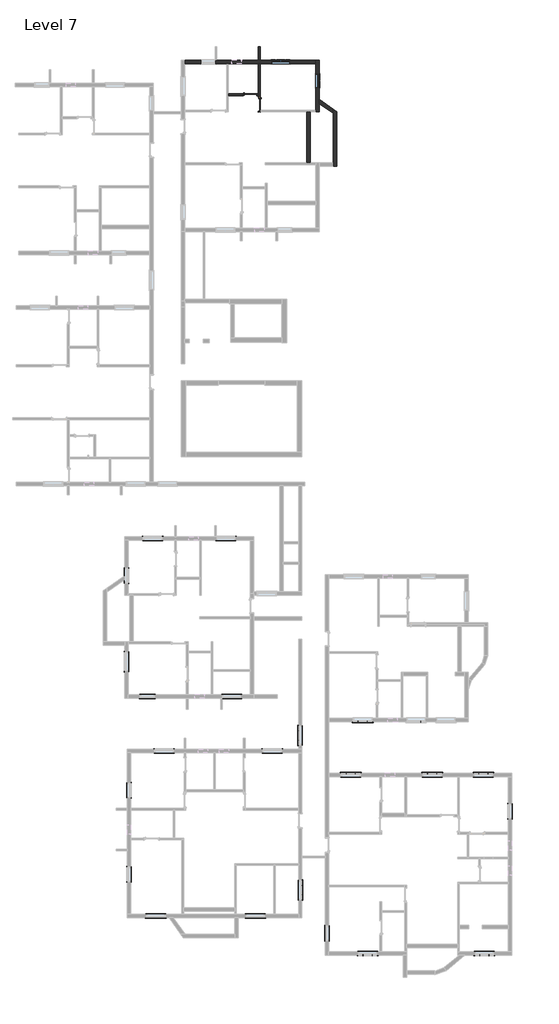
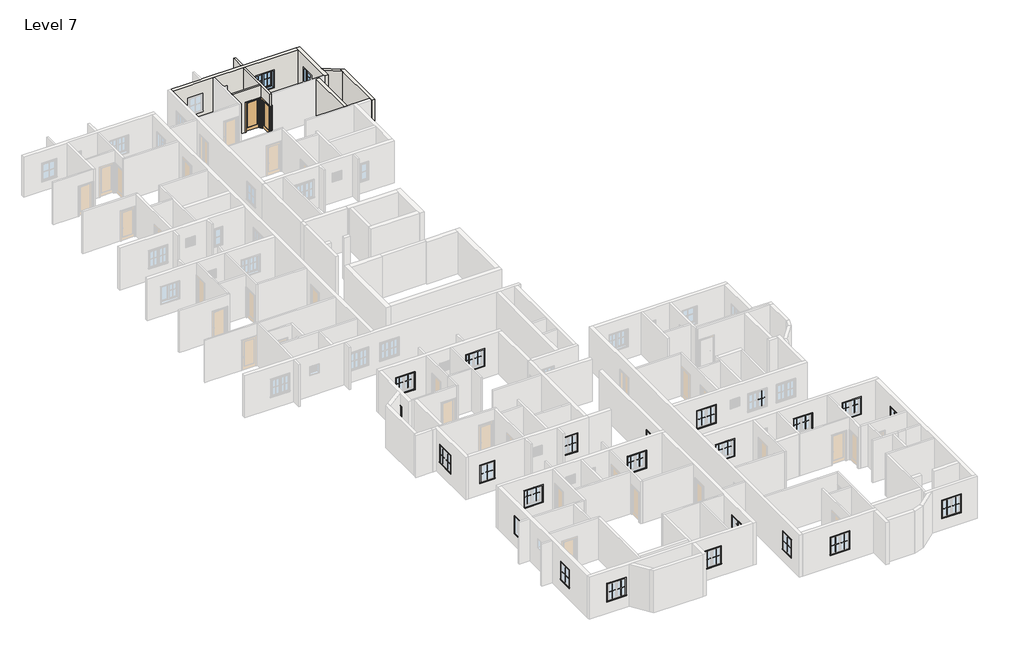
# One storey, part 6 of 7: 82 proxies, 8 walls, 2 doors, 2 windows.
"""IFC4 building model written with IfcOpenShell, lengths in millimetres."""

from ifc_helpers import new_model, si_unit, frame, origin, place, context, project, spatial, polyline, outline, extrude, faceted_brep, transform, mapped, element, save
from components import muntin_pattern_2x2_muntin_pattern_2x2_95b57395, muntin_pattern_2x2_muntin_pattern_2x2_4dfeb3f3, muntin_pattern_2x2_muntin_pattern_2x2_e852a7e4, trim_window_exterior_flat_with_sill_e4b28ec3, trim_window_exterior_flat_with_sill_7cfdd449, trim_window_interior_flat_picture_frame_39ff4276, trim_window_interior_flat_picture_frame_f1e0b15b, door_3c6ab76a, window_272f20d6, window_casement_double_4_x_4_af3140d2

model = new_model("IFC4")

# Units and contexts
model_context = context("Model", 3, world=origin())
ifc_project = project(units=[si_unit("LENGTHUNIT", "METRE", prefix="MILLI")], contexts=[model_context])

# Site, building, storey
site = spatial("IfcSite", under=ifc_project)
building = spatial("IfcBuilding", under=site)
storey = spatial("IfcBuildingStorey", under=building, Name="Level 7", Elevation=9601.2)

# Proxies
placement = place(None, origin())
muntin_pattern_2x2_muntin_pattern_2x2_shape = muntin_pattern_2x2_muntin_pattern_2x2_95b57395(model_context)
element("IfcBuildingElementProxy", 1, Name="Muntin Pattern_2x2 : Muntin Pattern_2x2", ObjectType="Muntin Pattern_2x2 : Muntin Pattern_2x2", at=placement, inside=storey, context=model_context, shape_type="MappedRepresentation", body=[
    mapped(muntin_pattern_2x2_muntin_pattern_2x2_shape, transform((17627.3240531, -20041.5997229, 10585.45), x_axis=(0.0, 1.0, 0.0), y_axis=(-1.0, 0.0, 0.0), z_axis=(0.0, 0.0, 1.0))),
])
element("IfcBuildingElementProxy", 2, Name="Muntin Pattern_2x2 : Muntin Pattern_2x2", ObjectType="Muntin Pattern_2x2 : Muntin Pattern_2x2", at=placement, inside=storey, context=model_context, shape_type="MappedRepresentation", body=[
    mapped(muntin_pattern_2x2_muntin_pattern_2x2_shape, transform((5625.8240531, -28048.9497229, 10585.45), x_axis=(0.0, 1.0, 0.0), y_axis=(-1.0, 0.0, 0.0), z_axis=(0.0, 0.0, 1.0))),
])
element("IfcBuildingElementProxy", 3, Name="Muntin Pattern_2x2 : Muntin Pattern_2x2", ObjectType="Muntin Pattern_2x2 : Muntin Pattern_2x2", at=placement, inside=storey, context=model_context, shape_type="MappedRepresentation", body=[
    mapped(muntin_pattern_2x2_muntin_pattern_2x2_shape, transform((-7378.9759469, -24172.9363256, 10585.45), x_axis=(0.0, 1.0, 0.0), y_axis=(-1.0, 0.0, 0.0), z_axis=(0.0, 0.0, 1.0))),
])
element("IfcBuildingElementProxy", 4, Name="Muntin Pattern_2x2 : Muntin Pattern_2x2", ObjectType="Muntin Pattern_2x2 : Muntin Pattern_2x2", at=placement, inside=storey, context=model_context, shape_type="MappedRepresentation", body=[
    mapped(muntin_pattern_2x2_muntin_pattern_2x2_shape, transform((-7169.4259469, -18656.0038828, 10585.45), x_axis=(0.0, -1.0, 0.0), y_axis=(1.0, 0.0, 0.0), z_axis=(0.0, 0.0, 1.0))),
])
element("IfcBuildingElementProxy", 5, Name="Muntin Pattern_2x2 : Muntin Pattern_2x2", ObjectType="Muntin Pattern_2x2 : Muntin Pattern_2x2", at=placement, inside=storey, context=model_context, shape_type="MappedRepresentation", body=[
    mapped(muntin_pattern_2x2_muntin_pattern_2x2_shape, transform((-6067.7009469, -12594.9288828, 10585.45), x_axis=(-1.0, 0.0, 0.0), y_axis=(0.0, -1.0, 0.0), z_axis=(0.0, 0.0, 1.0))),
])
element("IfcBuildingElementProxy", 6, Name="Muntin Pattern_2x2 : Muntin Pattern_2x2", ObjectType="Muntin Pattern_2x2 : Muntin Pattern_2x2", at=placement, inside=storey, context=model_context, shape_type="MappedRepresentation", body=[
    mapped(muntin_pattern_2x2_muntin_pattern_2x2_shape, transform((-7334.5259469, -4559.0038828, 10585.45), x_axis=(0.0, -1.0, 0.0), y_axis=(1.0, 0.0, 0.0), z_axis=(0.0, 0.0, 1.0))),
])
muntin_pattern_2x2_muntin_pattern_2x2_2_shape = muntin_pattern_2x2_muntin_pattern_2x2_4dfeb3f3(model_context)
element("IfcBuildingElementProxy", 7, Name="Muntin Pattern_2x2 : Muntin Pattern_2x2", ObjectType="Muntin Pattern_2x2 : Muntin Pattern_2x2", at=placement, inside=storey, context=model_context, shape_type="MappedRepresentation", body=[
    mapped(muntin_pattern_2x2_muntin_pattern_2x2_2_shape, transform((11869.4615531, -14158.3247229, 10585.45), x_axis=(-1.0, 0.0, 0.0), y_axis=(0.0, -1.0, 0.0), z_axis=(0.0, 0.0, 1.0))),
])
element("IfcBuildingElementProxy", 8, Name="Muntin Pattern_2x2 : Muntin Pattern_2x2", ObjectType="Muntin Pattern_2x2 : Muntin Pattern_2x2", at=placement, inside=storey, context=model_context, shape_type="MappedRepresentation", body=[
    mapped(muntin_pattern_2x2_muntin_pattern_2x2_2_shape, transform((8364.2615531, -14158.3247229, 10585.45), x_axis=(-1.0, 0.0, 0.0), y_axis=(0.0, -1.0, 0.0), z_axis=(0.0, 0.0, 1.0))),
])
element("IfcBuildingElementProxy", 9, Name="Muntin Pattern_2x2 : Muntin Pattern_2x2", ObjectType="Muntin Pattern_2x2 : Muntin Pattern_2x2", at=placement, inside=storey, context=model_context, shape_type="MappedRepresentation", body=[
    mapped(muntin_pattern_2x2_muntin_pattern_2x2_2_shape, transform((6976.7865531, -17530.1747229, 10585.45), x_axis=(1.0, 0.0, 0.0), y_axis=(0.0, 1.0, 0.0), z_axis=(0.0, 0.0, 1.0))),
])
element("IfcBuildingElementProxy", 10, Name="Muntin Pattern_2x2 : Muntin Pattern_2x2", ObjectType="Muntin Pattern_2x2 : Muntin Pattern_2x2", at=placement, inside=storey, context=model_context, shape_type="MappedRepresentation", body=[
    mapped(muntin_pattern_2x2_muntin_pattern_2x2_2_shape, transform((12323.4865531, -17530.1747229, 10585.45), x_axis=(1.0, 0.0, 0.0), y_axis=(0.0, 1.0, 0.0), z_axis=(0.0, 0.0, 1.0))),
])
element("IfcBuildingElementProxy", 11, Name="Muntin Pattern_2x2 : Muntin Pattern_2x2", ObjectType="Muntin Pattern_2x2 : Muntin Pattern_2x2", at=placement, inside=storey, context=model_context, shape_type="MappedRepresentation", body=[
    mapped(muntin_pattern_2x2_muntin_pattern_2x2_2_shape, transform((15682.6365531, -17530.1747229, 10585.45), x_axis=(1.0, 0.0, 0.0), y_axis=(0.0, 1.0, 0.0), z_axis=(0.0, 0.0, 1.0))),
])
element("IfcBuildingElementProxy", 12, Name="Muntin Pattern_2x2 : Muntin Pattern_2x2", ObjectType="Muntin Pattern_2x2 : Muntin Pattern_2x2", at=placement, inside=storey, context=model_context, shape_type="MappedRepresentation", body=[
    mapped(muntin_pattern_2x2_muntin_pattern_2x2_2_shape, transform((16349.3865531, -29474.5247229, 10585.45), x_axis=(-1.0, 0.0, 0.0), y_axis=(0.0, -1.0, 0.0), z_axis=(0.0, 0.0, 1.0))),
])
element("IfcBuildingElementProxy", 13, Name="Muntin Pattern_2x2 : Muntin Pattern_2x2", ObjectType="Muntin Pattern_2x2 : Muntin Pattern_2x2", at=placement, inside=storey, context=model_context, shape_type="MappedRepresentation", body=[
    mapped(muntin_pattern_2x2_muntin_pattern_2x2_2_shape, transform((8694.4615531, -29474.5247229, 10585.45), x_axis=(-1.0, 0.0, 0.0), y_axis=(0.0, -1.0, 0.0), z_axis=(0.0, 0.0, 1.0))),
])
element("IfcBuildingElementProxy", 14, Name="Muntin Pattern_2x2 : Muntin Pattern_2x2", ObjectType="Muntin Pattern_2x2 : Muntin Pattern_2x2", at=placement, inside=storey, context=model_context, shape_type="MappedRepresentation", body=[
    mapped(muntin_pattern_2x2_muntin_pattern_2x2_2_shape, transform((4070.0740531, -24902.8163828, 10585.45), x_axis=(0.0, -1.0, 0.0), y_axis=(1.0, 0.0, 0.0), z_axis=(0.0, 0.0, 1.0))),
])
element("IfcBuildingElementProxy", 15, Name="Muntin Pattern_2x2 : Muntin Pattern_2x2", ObjectType="Muntin Pattern_2x2 : Muntin Pattern_2x2", at=placement, inside=storey, context=model_context, shape_type="MappedRepresentation", body=[
    mapped(muntin_pattern_2x2_muntin_pattern_2x2_2_shape, transform((1325.2865531, -26996.7288828, 10585.45), x_axis=(-1.0, 0.0, 0.0), y_axis=(0.0, -1.0, 0.0), z_axis=(0.0, 0.0, 1.0))),
])
element("IfcBuildingElementProxy", 16, Name="Muntin Pattern_2x2 : Muntin Pattern_2x2", ObjectType="Muntin Pattern_2x2 : Muntin Pattern_2x2", at=placement, inside=storey, context=model_context, shape_type="MappedRepresentation", body=[
    mapped(muntin_pattern_2x2_muntin_pattern_2x2_2_shape, transform((-5208.8634469, -26996.7288828, 10585.45), x_axis=(-1.0, 0.0, 0.0), y_axis=(0.0, -1.0, 0.0), z_axis=(0.0, 0.0, 1.0))),
])
element("IfcBuildingElementProxy", 17, Name="Muntin Pattern_2x2 : Muntin Pattern_2x2", ObjectType="Muntin Pattern_2x2 : Muntin Pattern_2x2", at=placement, inside=storey, context=model_context, shape_type="MappedRepresentation", body=[
    mapped(muntin_pattern_2x2_muntin_pattern_2x2_2_shape, transform((1823.7615531, -15966.7788828, 10585.45), x_axis=(1.0, 0.0, 0.0), y_axis=(0.0, 1.0, 0.0), z_axis=(0.0, 0.0, 1.0))),
])
element("IfcBuildingElementProxy", 18, Name="Muntin Pattern_2x2 : Muntin Pattern_2x2", ObjectType="Muntin Pattern_2x2 : Muntin Pattern_2x2", at=placement, inside=storey, context=model_context, shape_type="MappedRepresentation", body=[
    mapped(muntin_pattern_2x2_muntin_pattern_2x2_2_shape, transform((-5272.3634469, -15966.7788828, 10585.45), x_axis=(1.0, 0.0, 0.0), y_axis=(0.0, 1.0, 0.0), z_axis=(0.0, 0.0, 1.0))),
])
element("IfcBuildingElementProxy", 19, Name="Muntin Pattern_2x2 : Muntin Pattern_2x2", ObjectType="Muntin Pattern_2x2 : Muntin Pattern_2x2", at=placement, inside=storey, context=model_context, shape_type="MappedRepresentation", body=[
    mapped(muntin_pattern_2x2_muntin_pattern_2x2_2_shape, transform((3860.5240531, -15358.7663828, 10585.45), x_axis=(0.0, 1.0, 0.0), y_axis=(-1.0, 0.0, 0.0), z_axis=(0.0, 0.0, 1.0))),
])
element("IfcBuildingElementProxy", 20, Name="Muntin Pattern_2x2 : Muntin Pattern_2x2", ObjectType="Muntin Pattern_2x2 : Muntin Pattern_2x2", at=placement, inside=storey, context=model_context, shape_type="MappedRepresentation", body=[
    mapped(muntin_pattern_2x2_muntin_pattern_2x2_2_shape, transform((-239.9884469, -12594.9288828, 10585.45), x_axis=(-1.0, 0.0, 0.0), y_axis=(0.0, -1.0, 0.0), z_axis=(0.0, 0.0, 1.0))),
])
element("IfcBuildingElementProxy", 21, Name="Muntin Pattern_2x2 : Muntin Pattern_2x2", ObjectType="Muntin Pattern_2x2 : Muntin Pattern_2x2", at=placement, inside=storey, context=model_context, shape_type="MappedRepresentation", body=[
    mapped(muntin_pattern_2x2_muntin_pattern_2x2_2_shape, transform((-7544.0759469, -10513.7163828, 10585.45), x_axis=(0.0, 1.0, 0.0), y_axis=(-1.0, 0.0, 0.0), z_axis=(0.0, 0.0, 1.0))),
])
element("IfcBuildingElementProxy", 22, Name="Muntin Pattern_2x2 : Muntin Pattern_2x2", ObjectType="Muntin Pattern_2x2 : Muntin Pattern_2x2", at=placement, inside=storey, context=model_context, shape_type="MappedRepresentation", body=[
    mapped(muntin_pattern_2x2_muntin_pattern_2x2_2_shape, transform((-6021.6634469, -2022.1788828, 10585.45), x_axis=(1.0, 0.0, 0.0), y_axis=(0.0, 1.0, 0.0), z_axis=(0.0, 0.0, 1.0))),
])
element("IfcBuildingElementProxy", 23, Name="Muntin Pattern_2x2 : Muntin Pattern_2x2", ObjectType="Muntin Pattern_2x2 : Muntin Pattern_2x2", at=placement, inside=storey, context=model_context, shape_type="MappedRepresentation", body=[
    mapped(muntin_pattern_2x2_muntin_pattern_2x2_2_shape, transform((-1221.0634469, -2022.1788828, 10585.45), x_axis=(1.0, 0.0, 0.0), y_axis=(0.0, 1.0, 0.0), z_axis=(0.0, 0.0, 1.0))),
])
muntin_pattern_2x2_muntin_pattern_2x2_3_shape = muntin_pattern_2x2_muntin_pattern_2x2_e852a7e4(model_context)
element("IfcBuildingElementProxy", 24, Name="Muntin Pattern_2x2 : Muntin Pattern_2x2", ObjectType="Muntin Pattern_2x2 : Muntin Pattern_2x2", at=placement, inside=storey, context=model_context, shape_type="MappedRepresentation", body=[
    mapped(muntin_pattern_2x2_muntin_pattern_2x2_3_shape, transform((7757.8365531, -14158.3247229, 10585.45), x_axis=(1.0, 0.0, 0.0), y_axis=(0.0, 1.0, 0.0), z_axis=(0.0, 0.0, 1.0))),
])
element("IfcBuildingElementProxy", 25, Name="Muntin Pattern_2x2 : Muntin Pattern_2x2", ObjectType="Muntin Pattern_2x2 : Muntin Pattern_2x2", at=placement, inside=storey, context=model_context, shape_type="MappedRepresentation", body=[
    mapped(muntin_pattern_2x2_muntin_pattern_2x2_3_shape, transform((7583.2115531, -17530.1747229, 10585.45), x_axis=(-1.0, 0.0, 0.0), y_axis=(0.0, -1.0, 0.0), z_axis=(0.0, 0.0, 1.0))),
])
element("IfcBuildingElementProxy", 26, Name="Muntin Pattern_2x2 : Muntin Pattern_2x2", ObjectType="Muntin Pattern_2x2 : Muntin Pattern_2x2", at=placement, inside=storey, context=model_context, shape_type="MappedRepresentation", body=[
    mapped(muntin_pattern_2x2_muntin_pattern_2x2_3_shape, transform((12929.9115531, -17530.1747229, 10585.45), x_axis=(-1.0, 0.0, 0.0), y_axis=(0.0, -1.0, 0.0), z_axis=(0.0, 0.0, 1.0))),
])
element("IfcBuildingElementProxy", 27, Name="Muntin Pattern_2x2 : Muntin Pattern_2x2", ObjectType="Muntin Pattern_2x2 : Muntin Pattern_2x2", at=placement, inside=storey, context=model_context, shape_type="MappedRepresentation", body=[
    mapped(muntin_pattern_2x2_muntin_pattern_2x2_3_shape, transform((16289.0615531, -17530.1747229, 10585.45), x_axis=(-1.0, 0.0, 0.0), y_axis=(0.0, -1.0, 0.0), z_axis=(0.0, 0.0, 1.0))),
])
element("IfcBuildingElementProxy", 28, Name="Muntin Pattern_2x2 : Muntin Pattern_2x2", ObjectType="Muntin Pattern_2x2 : Muntin Pattern_2x2", at=placement, inside=storey, context=model_context, shape_type="MappedRepresentation", body=[
    mapped(muntin_pattern_2x2_muntin_pattern_2x2_3_shape, transform((15742.9615531, -29474.5247229, 10585.45), x_axis=(1.0, 0.0, 0.0), y_axis=(0.0, 1.0, 0.0), z_axis=(0.0, 0.0, 1.0))),
])
element("IfcBuildingElementProxy", 29, Name="Muntin Pattern_2x2 : Muntin Pattern_2x2", ObjectType="Muntin Pattern_2x2 : Muntin Pattern_2x2", at=placement, inside=storey, context=model_context, shape_type="MappedRepresentation", body=[
    mapped(muntin_pattern_2x2_muntin_pattern_2x2_3_shape, transform((8088.0365531, -29474.5247229, 10585.45), x_axis=(1.0, 0.0, 0.0), y_axis=(0.0, 1.0, 0.0), z_axis=(0.0, 0.0, 1.0))),
])
element("IfcBuildingElementProxy", 30, Name="Muntin Pattern_2x2 : Muntin Pattern_2x2", ObjectType="Muntin Pattern_2x2 : Muntin Pattern_2x2", at=placement, inside=storey, context=model_context, shape_type="MappedRepresentation", body=[
    mapped(muntin_pattern_2x2_muntin_pattern_2x2_3_shape, transform((4070.0740531, -25509.2413828, 10585.45), x_axis=(0.0, 1.0, 0.0), y_axis=(-1.0, 0.0, 0.0), z_axis=(0.0, 0.0, 1.0))),
])
element("IfcBuildingElementProxy", 31, Name="Muntin Pattern_2x2 : Muntin Pattern_2x2", ObjectType="Muntin Pattern_2x2 : Muntin Pattern_2x2", at=placement, inside=storey, context=model_context, shape_type="MappedRepresentation", body=[
    mapped(muntin_pattern_2x2_muntin_pattern_2x2_3_shape, transform((718.8615531, -26996.7288828, 10585.45), x_axis=(1.0, 0.0, 0.0), y_axis=(0.0, 1.0, 0.0), z_axis=(0.0, 0.0, 1.0))),
])
element("IfcBuildingElementProxy", 32, Name="Muntin Pattern_2x2 : Muntin Pattern_2x2", ObjectType="Muntin Pattern_2x2 : Muntin Pattern_2x2", at=placement, inside=storey, context=model_context, shape_type="MappedRepresentation", body=[
    mapped(muntin_pattern_2x2_muntin_pattern_2x2_3_shape, transform((-5815.2884469, -26996.7288828, 10585.45), x_axis=(1.0, 0.0, 0.0), y_axis=(0.0, 1.0, 0.0), z_axis=(0.0, 0.0, 1.0))),
])
element("IfcBuildingElementProxy", 33, Name="Muntin Pattern_2x2 : Muntin Pattern_2x2", ObjectType="Muntin Pattern_2x2 : Muntin Pattern_2x2", at=placement, inside=storey, context=model_context, shape_type="MappedRepresentation", body=[
    mapped(muntin_pattern_2x2_muntin_pattern_2x2_3_shape, transform((2430.1865531, -15966.7788828, 10585.45), x_axis=(-1.0, 0.0, 0.0), y_axis=(0.0, -1.0, 0.0), z_axis=(0.0, 0.0, 1.0))),
])
element("IfcBuildingElementProxy", 34, Name="Muntin Pattern_2x2 : Muntin Pattern_2x2", ObjectType="Muntin Pattern_2x2 : Muntin Pattern_2x2", at=placement, inside=storey, context=model_context, shape_type="MappedRepresentation", body=[
    mapped(muntin_pattern_2x2_muntin_pattern_2x2_3_shape, transform((-4665.9384469, -15966.7788828, 10585.45), x_axis=(-1.0, 0.0, 0.0), y_axis=(0.0, -1.0, 0.0), z_axis=(0.0, 0.0, 1.0))),
])
element("IfcBuildingElementProxy", 35, Name="Muntin Pattern_2x2 : Muntin Pattern_2x2", ObjectType="Muntin Pattern_2x2 : Muntin Pattern_2x2", at=placement, inside=storey, context=model_context, shape_type="MappedRepresentation", body=[
    mapped(muntin_pattern_2x2_muntin_pattern_2x2_3_shape, transform((3860.5240531, -14752.3413828, 10585.45), x_axis=(0.0, -1.0, 0.0), y_axis=(1.0, 0.0, 0.0), z_axis=(0.0, 0.0, 1.0))),
])
element("IfcBuildingElementProxy", 36, Name="Muntin Pattern_2x2 : Muntin Pattern_2x2", ObjectType="Muntin Pattern_2x2 : Muntin Pattern_2x2", at=placement, inside=storey, context=model_context, shape_type="MappedRepresentation", body=[
    mapped(muntin_pattern_2x2_muntin_pattern_2x2_3_shape, transform((-846.4134469, -12594.9288828, 10585.45), x_axis=(1.0, 0.0, 0.0), y_axis=(0.0, 1.0, 0.0), z_axis=(0.0, 0.0, 1.0))),
])
element("IfcBuildingElementProxy", 37, Name="Muntin Pattern_2x2 : Muntin Pattern_2x2", ObjectType="Muntin Pattern_2x2 : Muntin Pattern_2x2", at=placement, inside=storey, context=model_context, shape_type="MappedRepresentation", body=[
    mapped(muntin_pattern_2x2_muntin_pattern_2x2_3_shape, transform((-7544.0759469, -9907.2913828, 10585.45), x_axis=(0.0, -1.0, 0.0), y_axis=(1.0, 0.0, 0.0), z_axis=(0.0, 0.0, 1.0))),
])
element("IfcBuildingElementProxy", 38, Name="Muntin Pattern_2x2 : Muntin Pattern_2x2", ObjectType="Muntin Pattern_2x2 : Muntin Pattern_2x2", at=placement, inside=storey, context=model_context, shape_type="MappedRepresentation", body=[
    mapped(muntin_pattern_2x2_muntin_pattern_2x2_3_shape, transform((-5415.2384469, -2022.1788828, 10585.45), x_axis=(-1.0, 0.0, 0.0), y_axis=(0.0, -1.0, 0.0), z_axis=(0.0, 0.0, 1.0))),
])
element("IfcBuildingElementProxy", 39, Name="Muntin Pattern_2x2 : Muntin Pattern_2x2", ObjectType="Muntin Pattern_2x2 : Muntin Pattern_2x2", at=placement, inside=storey, context=model_context, shape_type="MappedRepresentation", body=[
    mapped(muntin_pattern_2x2_muntin_pattern_2x2_3_shape, transform((-614.6384469, -2022.1788828, 10585.45), x_axis=(-1.0, 0.0, 0.0), y_axis=(0.0, -1.0, 0.0), z_axis=(0.0, 0.0, 1.0))),
])
trim_window_exterior_flat_with_sill_shape = trim_window_exterior_flat_with_sill_e4b28ec3(model_context)
element("IfcBuildingElementProxy", 40, Name="Trim-Window-Exterior-Flat : with Sill", ObjectType="Trim-Window-Exterior-Flat : with Sill", at=placement, inside=storey, context=model_context, shape_type="MappedRepresentation", body=[
    mapped(trim_window_exterior_flat_with_sill_shape, transform((17617.7990531, -20041.5997229, 11734.8), x_axis=(0.0, -1.0, 0.0), y_axis=(0.0, 0.0, 1.0), z_axis=(-1.0, 0.0, 0.0))),
])
element("IfcBuildingElementProxy", 41, Name="Trim-Window-Exterior-Flat : with Sill", ObjectType="Trim-Window-Exterior-Flat : with Sill", at=placement, inside=storey, context=model_context, shape_type="MappedRepresentation", body=[
    mapped(trim_window_exterior_flat_with_sill_shape, transform((5616.2990531, -28048.9497229, 11734.8), x_axis=(0.0, -1.0, 0.0), y_axis=(0.0, 0.0, 1.0), z_axis=(-1.0, 0.0, 0.0))),
])
element("IfcBuildingElementProxy", 42, Name="Trim-Window-Exterior-Flat : with Sill", ObjectType="Trim-Window-Exterior-Flat : with Sill", at=placement, inside=storey, context=model_context, shape_type="MappedRepresentation", body=[
    mapped(trim_window_exterior_flat_with_sill_shape, transform((-7388.5009469, -24172.9363256, 11734.8), x_axis=(0.0, -1.0, 0.0), y_axis=(0.0, 0.0, 1.0), z_axis=(-1.0, 0.0, 0.0))),
])
element("IfcBuildingElementProxy", 43, Name="Trim-Window-Exterior-Flat : with Sill", ObjectType="Trim-Window-Exterior-Flat : with Sill", at=placement, inside=storey, context=model_context, shape_type="MappedRepresentation", body=[
    mapped(trim_window_exterior_flat_with_sill_shape, transform((-7159.9009469, -18656.0038828, 11734.8), x_axis=(0.0, 1.0, 0.0), y_axis=(0.0, 0.0, 1.0), z_axis=(1.0, 0.0, 0.0))),
])
element("IfcBuildingElementProxy", 44, Name="Trim-Window-Exterior-Flat : with Sill", ObjectType="Trim-Window-Exterior-Flat : with Sill", at=placement, inside=storey, context=model_context, shape_type="MappedRepresentation", body=[
    mapped(trim_window_exterior_flat_with_sill_shape, transform((-6067.7009469, -12604.4538828, 11734.8), x_axis=(1.0, 0.0, 0.0), y_axis=(0.0, 0.0, 1.0), z_axis=(0.0, -1.0, 0.0))),
])
element("IfcBuildingElementProxy", 45, Name="Trim-Window-Exterior-Flat : with Sill", ObjectType="Trim-Window-Exterior-Flat : with Sill", at=placement, inside=storey, context=model_context, shape_type="MappedRepresentation", body=[
    mapped(trim_window_exterior_flat_with_sill_shape, transform((-7325.0009469, -4559.0038828, 11734.8), x_axis=(0.0, 1.0, 0.0), y_axis=(0.0, 0.0, 1.0), z_axis=(1.0, 0.0, 0.0))),
])
trim_window_exterior_flat_with_sill_2_shape = trim_window_exterior_flat_with_sill_7cfdd449(model_context)
element("IfcBuildingElementProxy", 46, Name="Trim-Window-Exterior-Flat : with Sill", ObjectType="Trim-Window-Exterior-Flat : with Sill", at=placement, inside=storey, context=model_context, shape_type="MappedRepresentation", body=[
    mapped(trim_window_exterior_flat_with_sill_2_shape, transform((8061.0490531, -14167.8497229, 11734.8), x_axis=(1.0, 0.0, 0.0), y_axis=(0.0, 0.0, 1.0), z_axis=(0.0, -1.0, 0.0))),
])
element("IfcBuildingElementProxy", 47, Name="Trim-Window-Exterior-Flat : with Sill", ObjectType="Trim-Window-Exterior-Flat : with Sill", at=placement, inside=storey, context=model_context, shape_type="MappedRepresentation", body=[
    mapped(trim_window_exterior_flat_with_sill_2_shape, transform((7279.9990531, -17520.6497229, 11734.8), x_axis=(-1.0, 0.0, 0.0), y_axis=(0.0, 0.0, 1.0), z_axis=(0.0, 1.0, 0.0))),
])
element("IfcBuildingElementProxy", 48, Name="Trim-Window-Exterior-Flat : with Sill", ObjectType="Trim-Window-Exterior-Flat : with Sill", at=placement, inside=storey, context=model_context, shape_type="MappedRepresentation", body=[
    mapped(trim_window_exterior_flat_with_sill_2_shape, transform((12626.6990531, -17520.6497229, 11734.8), x_axis=(-1.0, 0.0, 0.0), y_axis=(0.0, 0.0, 1.0), z_axis=(0.0, 1.0, 0.0))),
])
element("IfcBuildingElementProxy", 49, Name="Trim-Window-Exterior-Flat : with Sill", ObjectType="Trim-Window-Exterior-Flat : with Sill", at=placement, inside=storey, context=model_context, shape_type="MappedRepresentation", body=[
    mapped(trim_window_exterior_flat_with_sill_2_shape, transform((15985.8490531, -17520.6497229, 11734.8), x_axis=(-1.0, 0.0, 0.0), y_axis=(0.0, 0.0, 1.0), z_axis=(0.0, 1.0, 0.0))),
])
element("IfcBuildingElementProxy", 50, Name="Trim-Window-Exterior-Flat : with Sill", ObjectType="Trim-Window-Exterior-Flat : with Sill", at=placement, inside=storey, context=model_context, shape_type="MappedRepresentation", body=[
    mapped(trim_window_exterior_flat_with_sill_2_shape, transform((16046.1740531, -29484.0497229, 11734.8), x_axis=(1.0, 0.0, 0.0), y_axis=(0.0, 0.0, 1.0), z_axis=(0.0, -1.0, 0.0))),
])
element("IfcBuildingElementProxy", 51, Name="Trim-Window-Exterior-Flat : with Sill", ObjectType="Trim-Window-Exterior-Flat : with Sill", at=placement, inside=storey, context=model_context, shape_type="MappedRepresentation", body=[
    mapped(trim_window_exterior_flat_with_sill_2_shape, transform((8391.2490531, -29484.0497229, 11734.8), x_axis=(1.0, 0.0, 0.0), y_axis=(0.0, 0.0, 1.0), z_axis=(0.0, -1.0, 0.0))),
])
element("IfcBuildingElementProxy", 52, Name="Trim-Window-Exterior-Flat : with Sill", ObjectType="Trim-Window-Exterior-Flat : with Sill", at=placement, inside=storey, context=model_context, shape_type="MappedRepresentation", body=[
    mapped(trim_window_exterior_flat_with_sill_2_shape, transform((4079.5990531, -25206.0288828, 11734.8), x_axis=(0.0, 1.0, 0.0), y_axis=(0.0, 0.0, 1.0), z_axis=(1.0, 0.0, 0.0))),
])
element("IfcBuildingElementProxy", 53, Name="Trim-Window-Exterior-Flat : with Sill", ObjectType="Trim-Window-Exterior-Flat : with Sill", at=placement, inside=storey, context=model_context, shape_type="MappedRepresentation", body=[
    mapped(trim_window_exterior_flat_with_sill_2_shape, transform((1022.0740531, -27006.2538828, 11734.8), x_axis=(1.0, 0.0, 0.0), y_axis=(0.0, 0.0, 1.0), z_axis=(0.0, -1.0, 0.0))),
])
element("IfcBuildingElementProxy", 54, Name="Trim-Window-Exterior-Flat : with Sill", ObjectType="Trim-Window-Exterior-Flat : with Sill", at=placement, inside=storey, context=model_context, shape_type="MappedRepresentation", body=[
    mapped(trim_window_exterior_flat_with_sill_2_shape, transform((-5512.0759469, -27006.2538828, 11734.8), x_axis=(1.0, 0.0, 0.0), y_axis=(0.0, 0.0, 1.0), z_axis=(0.0, -1.0, 0.0))),
])
element("IfcBuildingElementProxy", 55, Name="Trim-Window-Exterior-Flat : with Sill", ObjectType="Trim-Window-Exterior-Flat : with Sill", at=placement, inside=storey, context=model_context, shape_type="MappedRepresentation", body=[
    mapped(trim_window_exterior_flat_with_sill_2_shape, transform((2126.9740531, -15957.2538828, 11734.8), x_axis=(-1.0, 0.0, 0.0), y_axis=(0.0, 0.0, 1.0), z_axis=(0.0, 1.0, 0.0))),
])
element("IfcBuildingElementProxy", 56, Name="Trim-Window-Exterior-Flat : with Sill", ObjectType="Trim-Window-Exterior-Flat : with Sill", at=placement, inside=storey, context=model_context, shape_type="MappedRepresentation", body=[
    mapped(trim_window_exterior_flat_with_sill_2_shape, transform((-4969.1509469, -15957.2538828, 11734.8), x_axis=(-1.0, 0.0, 0.0), y_axis=(0.0, 0.0, 1.0), z_axis=(0.0, 1.0, 0.0))),
])
element("IfcBuildingElementProxy", 57, Name="Trim-Window-Exterior-Flat : with Sill", ObjectType="Trim-Window-Exterior-Flat : with Sill", at=placement, inside=storey, context=model_context, shape_type="MappedRepresentation", body=[
    mapped(trim_window_exterior_flat_with_sill_2_shape, transform((3850.9990531, -15055.5538828, 11734.8), x_axis=(0.0, -1.0, 0.0), y_axis=(0.0, 0.0, 1.0), z_axis=(-1.0, 0.0, 0.0))),
])
element("IfcBuildingElementProxy", 58, Name="Trim-Window-Exterior-Flat : with Sill", ObjectType="Trim-Window-Exterior-Flat : with Sill", at=placement, inside=storey, context=model_context, shape_type="MappedRepresentation", body=[
    mapped(trim_window_exterior_flat_with_sill_2_shape, transform((-543.2009469, -12604.4538828, 11734.8), x_axis=(1.0, 0.0, 0.0), y_axis=(0.0, 0.0, 1.0), z_axis=(0.0, -1.0, 0.0))),
])
element("IfcBuildingElementProxy", 59, Name="Trim-Window-Exterior-Flat : with Sill", ObjectType="Trim-Window-Exterior-Flat : with Sill", at=placement, inside=storey, context=model_context, shape_type="MappedRepresentation", body=[
    mapped(trim_window_exterior_flat_with_sill_2_shape, transform((-7553.6009469, -10210.5038828, 11734.8), x_axis=(0.0, -1.0, 0.0), y_axis=(0.0, 0.0, 1.0), z_axis=(-1.0, 0.0, 0.0))),
])
element("IfcBuildingElementProxy", 60, Name="Trim-Window-Exterior-Flat : with Sill", ObjectType="Trim-Window-Exterior-Flat : with Sill", at=placement, inside=storey, context=model_context, shape_type="MappedRepresentation", body=[
    mapped(trim_window_exterior_flat_with_sill_2_shape, transform((-5718.4509469, -2012.6538828, 11734.8), x_axis=(-1.0, 0.0, 0.0), y_axis=(0.0, 0.0, 1.0), z_axis=(0.0, 1.0, 0.0))),
])
element("IfcBuildingElementProxy", 61, Name="Trim-Window-Exterior-Flat : with Sill", ObjectType="Trim-Window-Exterior-Flat : with Sill", at=placement, inside=storey, context=model_context, shape_type="MappedRepresentation", body=[
    mapped(trim_window_exterior_flat_with_sill_2_shape, transform((-917.8509469, -2012.6538828, 11734.8), x_axis=(-1.0, 0.0, 0.0), y_axis=(0.0, 0.0, 1.0), z_axis=(0.0, 1.0, 0.0))),
])
trim_window_interior_flat_picture_frame_shape = trim_window_interior_flat_picture_frame_39ff4276(model_context)
element("IfcBuildingElementProxy", 62, Name="Trim-Window-Interior-Flat : Picture Frame", ObjectType="Trim-Window-Interior-Flat : Picture Frame", at=placement, inside=storey, context=model_context, shape_type="MappedRepresentation", body=[
    mapped(trim_window_interior_flat_picture_frame_shape, transform((17846.3990531, -20041.5997229, 11734.8), x_axis=(0.0, 1.0, 0.0), y_axis=(0.0, 0.0, 1.0), z_axis=(1.0, 0.0, 0.0))),
])
element("IfcBuildingElementProxy", 63, Name="Trim-Window-Interior-Flat : Picture Frame", ObjectType="Trim-Window-Interior-Flat : Picture Frame", at=placement, inside=storey, context=model_context, shape_type="MappedRepresentation", body=[
    mapped(trim_window_interior_flat_picture_frame_shape, transform((5844.8990531, -28048.9497229, 11734.8), x_axis=(0.0, 1.0, 0.0), y_axis=(0.0, 0.0, 1.0), z_axis=(1.0, 0.0, 0.0))),
])
element("IfcBuildingElementProxy", 64, Name="Trim-Window-Interior-Flat : Picture Frame", ObjectType="Trim-Window-Interior-Flat : Picture Frame", at=placement, inside=storey, context=model_context, shape_type="MappedRepresentation", body=[
    mapped(trim_window_interior_flat_picture_frame_shape, transform((-7159.9009469, -24172.9363256, 11734.8), x_axis=(0.0, 1.0, 0.0), y_axis=(0.0, 0.0, 1.0), z_axis=(1.0, 0.0, 0.0))),
])
element("IfcBuildingElementProxy", 65, Name="Trim-Window-Interior-Flat : Picture Frame", ObjectType="Trim-Window-Interior-Flat : Picture Frame", at=placement, inside=storey, context=model_context, shape_type="MappedRepresentation", body=[
    mapped(trim_window_interior_flat_picture_frame_shape, transform((-7388.5009469, -18656.0038828, 11734.8), x_axis=(0.0, -1.0, 0.0), y_axis=(0.0, 0.0, 1.0), z_axis=(-1.0, 0.0, 0.0))),
])
element("IfcBuildingElementProxy", 66, Name="Trim-Window-Interior-Flat : Picture Frame", ObjectType="Trim-Window-Interior-Flat : Picture Frame", at=placement, inside=storey, context=model_context, shape_type="MappedRepresentation", body=[
    mapped(trim_window_interior_flat_picture_frame_shape, transform((-6067.7009469, -12375.8538828, 11734.8), x_axis=(-1.0, 0.0, 0.0), y_axis=(0.0, 0.0, 1.0), z_axis=(0.0, 1.0, 0.0))),
])
element("IfcBuildingElementProxy", 67, Name="Trim-Window-Interior-Flat : Picture Frame", ObjectType="Trim-Window-Interior-Flat : Picture Frame", at=placement, inside=storey, context=model_context, shape_type="MappedRepresentation", body=[
    mapped(trim_window_interior_flat_picture_frame_shape, transform((-7553.6009469, -4559.0038828, 11734.8), x_axis=(0.0, -1.0, 0.0), y_axis=(0.0, 0.0, 1.0), z_axis=(-1.0, 0.0, 0.0))),
])
trim_window_interior_flat_picture_frame_2_shape = trim_window_interior_flat_picture_frame_f1e0b15b(model_context)
element("IfcBuildingElementProxy", 68, Name="Trim-Window-Interior-Flat : Picture Frame", ObjectType="Trim-Window-Interior-Flat : Picture Frame", at=placement, inside=storey, context=model_context, shape_type="MappedRepresentation", body=[
    mapped(trim_window_interior_flat_picture_frame_2_shape, transform((7279.9990531, -17749.2497229, 11734.8), x_axis=(1.0, 0.0, 0.0), y_axis=(0.0, 0.0, 1.0), z_axis=(0.0, -1.0, 0.0))),
])
element("IfcBuildingElementProxy", 69, Name="Trim-Window-Interior-Flat : Picture Frame", ObjectType="Trim-Window-Interior-Flat : Picture Frame", at=placement, inside=storey, context=model_context, shape_type="MappedRepresentation", body=[
    mapped(trim_window_interior_flat_picture_frame_2_shape, transform((12626.6990531, -17749.2497229, 11734.8), x_axis=(1.0, 0.0, 0.0), y_axis=(0.0, 0.0, 1.0), z_axis=(0.0, -1.0, 0.0))),
])
element("IfcBuildingElementProxy", 70, Name="Trim-Window-Interior-Flat : Picture Frame", ObjectType="Trim-Window-Interior-Flat : Picture Frame", at=placement, inside=storey, context=model_context, shape_type="MappedRepresentation", body=[
    mapped(trim_window_interior_flat_picture_frame_2_shape, transform((15985.8490531, -17749.2497229, 11734.8), x_axis=(1.0, 0.0, 0.0), y_axis=(0.0, 0.0, 1.0), z_axis=(0.0, -1.0, 0.0))),
])
element("IfcBuildingElementProxy", 71, Name="Trim-Window-Interior-Flat : Picture Frame", ObjectType="Trim-Window-Interior-Flat : Picture Frame", at=placement, inside=storey, context=model_context, shape_type="MappedRepresentation", body=[
    mapped(trim_window_interior_flat_picture_frame_2_shape, transform((16046.1740531, -29255.4497229, 11734.8), x_axis=(-1.0, 0.0, 0.0), y_axis=(0.0, 0.0, 1.0), z_axis=(0.0, 1.0, 0.0))),
])
element("IfcBuildingElementProxy", 72, Name="Trim-Window-Interior-Flat : Picture Frame", ObjectType="Trim-Window-Interior-Flat : Picture Frame", at=placement, inside=storey, context=model_context, shape_type="MappedRepresentation", body=[
    mapped(trim_window_interior_flat_picture_frame_2_shape, transform((8391.2490531, -29255.4497229, 11734.8), x_axis=(-1.0, 0.0, 0.0), y_axis=(0.0, 0.0, 1.0), z_axis=(0.0, 1.0, 0.0))),
])
element("IfcBuildingElementProxy", 73, Name="Trim-Window-Interior-Flat : Picture Frame", ObjectType="Trim-Window-Interior-Flat : Picture Frame", at=placement, inside=storey, context=model_context, shape_type="MappedRepresentation", body=[
    mapped(trim_window_interior_flat_picture_frame_2_shape, transform((3850.9990531, -25206.0288828, 11734.8), x_axis=(0.0, -1.0, 0.0), y_axis=(0.0, 0.0, 1.0), z_axis=(-1.0, 0.0, 0.0))),
])
element("IfcBuildingElementProxy", 74, Name="Trim-Window-Interior-Flat : Picture Frame", ObjectType="Trim-Window-Interior-Flat : Picture Frame", at=placement, inside=storey, context=model_context, shape_type="MappedRepresentation", body=[
    mapped(trim_window_interior_flat_picture_frame_2_shape, transform((1022.0740531, -26777.6538828, 11734.8), x_axis=(-1.0, 0.0, 0.0), y_axis=(0.0, 0.0, 1.0), z_axis=(0.0, 1.0, 0.0))),
])
element("IfcBuildingElementProxy", 75, Name="Trim-Window-Interior-Flat : Picture Frame", ObjectType="Trim-Window-Interior-Flat : Picture Frame", at=placement, inside=storey, context=model_context, shape_type="MappedRepresentation", body=[
    mapped(trim_window_interior_flat_picture_frame_2_shape, transform((-5512.0759469, -26777.6538828, 11734.8), x_axis=(-1.0, 0.0, 0.0), y_axis=(0.0, 0.0, 1.0), z_axis=(0.0, 1.0, 0.0))),
])
element("IfcBuildingElementProxy", 76, Name="Trim-Window-Interior-Flat : Picture Frame", ObjectType="Trim-Window-Interior-Flat : Picture Frame", at=placement, inside=storey, context=model_context, shape_type="MappedRepresentation", body=[
    mapped(trim_window_interior_flat_picture_frame_2_shape, transform((2126.9740531, -16185.8538828, 11734.8), x_axis=(1.0, 0.0, 0.0), y_axis=(0.0, 0.0, 1.0), z_axis=(0.0, -1.0, 0.0))),
])
element("IfcBuildingElementProxy", 77, Name="Trim-Window-Interior-Flat : Picture Frame", ObjectType="Trim-Window-Interior-Flat : Picture Frame", at=placement, inside=storey, context=model_context, shape_type="MappedRepresentation", body=[
    mapped(trim_window_interior_flat_picture_frame_2_shape, transform((-4969.1509469, -16185.8538828, 11734.8), x_axis=(1.0, 0.0, 0.0), y_axis=(0.0, 0.0, 1.0), z_axis=(0.0, -1.0, 0.0))),
])
element("IfcBuildingElementProxy", 78, Name="Trim-Window-Interior-Flat : Picture Frame", ObjectType="Trim-Window-Interior-Flat : Picture Frame", at=placement, inside=storey, context=model_context, shape_type="MappedRepresentation", body=[
    mapped(trim_window_interior_flat_picture_frame_2_shape, transform((4079.5990531, -15055.5538828, 11734.8), x_axis=(0.0, 1.0, 0.0), y_axis=(0.0, 0.0, 1.0), z_axis=(1.0, 0.0, 0.0))),
])
element("IfcBuildingElementProxy", 79, Name="Trim-Window-Interior-Flat : Picture Frame", ObjectType="Trim-Window-Interior-Flat : Picture Frame", at=placement, inside=storey, context=model_context, shape_type="MappedRepresentation", body=[
    mapped(trim_window_interior_flat_picture_frame_2_shape, transform((-543.2009469, -12375.8538828, 11734.8), x_axis=(-1.0, 0.0, 0.0), y_axis=(0.0, 0.0, 1.0), z_axis=(0.0, 1.0, 0.0))),
])
element("IfcBuildingElementProxy", 80, Name="Trim-Window-Interior-Flat : Picture Frame", ObjectType="Trim-Window-Interior-Flat : Picture Frame", at=placement, inside=storey, context=model_context, shape_type="MappedRepresentation", body=[
    mapped(trim_window_interior_flat_picture_frame_2_shape, transform((-7325.0009469, -10210.5038828, 11734.8), x_axis=(0.0, 1.0, 0.0), y_axis=(0.0, 0.0, 1.0), z_axis=(1.0, 0.0, 0.0))),
])
element("IfcBuildingElementProxy", 81, Name="Trim-Window-Interior-Flat : Picture Frame", ObjectType="Trim-Window-Interior-Flat : Picture Frame", at=placement, inside=storey, context=model_context, shape_type="MappedRepresentation", body=[
    mapped(trim_window_interior_flat_picture_frame_2_shape, transform((-5718.4509469, -2241.2538828, 11734.8), x_axis=(1.0, 0.0, 0.0), y_axis=(0.0, 0.0, 1.0), z_axis=(0.0, -1.0, 0.0))),
])
element("IfcBuildingElementProxy", 82, Name="Trim-Window-Interior-Flat : Picture Frame", ObjectType="Trim-Window-Interior-Flat : Picture Frame", at=placement, inside=storey, context=model_context, shape_type="MappedRepresentation", body=[
    mapped(trim_window_interior_flat_picture_frame_2_shape, transform((-917.8509469, -2241.2538828, 11734.8), x_axis=(1.0, 0.0, 0.0), y_axis=(0.0, 0.0, 1.0), z_axis=(0.0, -1.0, 0.0))),
])

# Doors
door_shape = door_3c6ab76a(model_context)
element("IfcDoor", 83, ObjectType="Door-Interior-Single-1_Panel-Wood : 2'6\" x 7' door", at=placement, inside=storey, context=model_context, shape_type="MappedRepresentation", body=[
    mapped(door_shape, transform((669.6490531, 27005.8505084, 9601.2), x_axis=(1.0, 0.0, 0.0), y_axis=(0.0, 1.0, 0.0), z_axis=(0.0, 0.0, 1.0))),
])
element("IfcDoor", 84, ObjectType="Door-Interior-Single-1_Panel-Wood : 36\" x 84\"", at=placement, inside=storey, context=model_context, shape_type="MappedRepresentation", body=[
    mapped(door_shape, transform((1282.4240531, 26367.6755084, 9601.2), x_axis=(0.0, -1.0, 0.0), y_axis=(1.0, 0.0, 0.0), z_axis=(0.0, 0.0, 1.0))),
])

# Walls
element("IfcWall", 85, ObjectType="4.5\" wall", at=placement, inside=storey, context=model_context, shape_type="Brep", body=[
    faceted_brep([(1336.3990531, 29041.0255084, 12649.2), (1336.3990531, 25993.0255084, 12649.2), (1336.3990531, 25878.7255084, 12649.2), (1336.3990531, 25878.7255084, 9601.2), (1336.3990531, 25885.0755084, 9601.2), (1336.3990531, 25885.0755084, 11760.2), (1336.3990531, 26850.2755084, 11760.2), (1336.3990531, 26850.2755084, 9601.2), (1336.3990531, 29041.0255084, 9601.2), (1222.0990531, 25878.7255084, 12649.2), (1222.0990531, 26945.5255084, 12649.2), (1222.0990531, 27059.8255084, 12649.2), (1222.0990531, 29041.0255084, 12649.2), (1222.0990531, 29041.0255084, 9601.2), (1222.0990531, 27059.8255084, 9601.2), (1222.0990531, 26945.5255084, 9601.2), (1222.0990531, 26850.2755084, 9601.2), (1222.0990531, 26850.2755084, 11760.2), (1222.0990531, 25885.0755084, 11760.2), (1222.0990531, 25885.0755084, 9601.2), (1222.0990531, 25878.7255084, 9601.2)], [[[0, 1, 2, 3, 4, 5, 6, 7, 8]], [[9, 10, 11, 12, 13, 14, 15, 16, 17, 18, 19, 20]], [[13, 8, 7, 16, 15, 14]], [[3, 20, 19, 4]], [[2, 1, 0, 12, 11, 10, 9]], [[0, 8, 13, 12]], [[3, 2, 9, 20]], [[18, 5, 4, 19]], [[5, 18, 17, 6]], [[6, 17, 16, 7]]]),
])
element("IfcWall", 86, ObjectType="4.5\" wall", at=placement, inside=storey, context=model_context, shape_type="SweptSolid", body=[
    extrude(outline(polyline([(12649.2, 1222.0990531), (12649.2, -759.1009469), (9601.2, -759.1009469), (9601.2, 187.0490531), (11760.2, 187.0490531), (11760.2, 1152.2490531), (9601.2, 1152.2490531), (9601.2, 1222.0990531), (12649.2, 1222.0990531)])), frame((0.0, 26945.5255084, 0.0), z_axis=(0.0, 1.0, 0.0), x_axis=(0.0, 0.0, 1.0)), (0.0, 0.0, 1.0), 114.3),
])
element("IfcWall", 87, ObjectType="4.5\" wall", at=placement, inside=storey, context=model_context, shape_type="SweptSolid", body=[
    extrude(outline(polyline([(1336.3990531, 30161.6889788), (1336.3990531, 29269.6255084), (1222.0990531, 29269.6255084), (1222.0990531, 30161.6889788), (1336.3990531, 30161.6889788)])), frame((0.0, 0.0, 9601.2), z_axis=(0.0, 0.0, 1.0), x_axis=(1.0, 0.0, 0.0)), (0.0, 0.0, 1.0), 3048.0),
])
element("IfcWall", 88, ObjectType="9\"", at=placement, inside=storey, context=model_context, shape_type="Brep", body=[
    faceted_brep([(-3616.6009469, 29041.0255084, 9601.2), (-873.4009469, 29041.0255084, 9601.2), (-759.1009469, 29041.0255084, 9601.2), (1222.0990531, 29041.0255084, 9601.2), (1336.3990531, 29041.0255084, 9601.2), (4993.9990531, 29041.0255084, 9601.2), (4993.9990531, 29041.0255084, 12649.2), (1336.3990531, 29041.0255084, 12649.2), (1222.0990531, 29041.0255084, 12649.2), (-759.1009469, 29041.0255084, 12649.2), (-873.4009469, 29041.0255084, 12649.2), (-3616.6009469, 29041.0255084, 12649.2), (91.7990531, 29041.0255084, 11734.8), (91.7990531, 29041.0255084, 11125.2), (-517.8009469, 29041.0255084, 11125.2), (-517.8009469, 29041.0255084, 11734.8), (-2532.2862554, 29041.0255084, 11734.8), (-1617.8862554, 29041.0255084, 11734.8), (-1617.8862554, 29041.0255084, 10515.6), (-2532.2862554, 29041.0255084, 10515.6), (3285.8490531, 29041.0255084, 11734.8), (3285.8490531, 29041.0255084, 10515.6), (2066.6490531, 29041.0255084, 10515.6), (2066.6490531, 29041.0255084, 11734.8), (-3616.6009469, 29269.6255084, 9601.2), (-3616.6009469, 29269.6255084, 12649.2), (-1617.8862554, 29269.6255084, 12649.2), (-1503.5862554, 29269.6255084, 12649.2), (1222.0990531, 29269.6255084, 12649.2), (1336.3990531, 29269.6255084, 12649.2), (4993.9990531, 29269.6255084, 12649.2), (4993.9990531, 29269.6255084, 9601.2), (1336.3990531, 29269.6255084, 9601.2), (1222.0990531, 29269.6255084, 9601.2), (-1503.5862554, 29269.6255084, 9601.2), (-1617.8862554, 29269.6255084, 9601.2), (91.7990531, 29269.6255084, 11734.8), (-517.8009469, 29269.6255084, 11734.8), (-517.8009469, 29269.6255084, 11125.2), (91.7990531, 29269.6255084, 11125.2), (-2532.2862554, 29269.6255084, 11734.8), (-2532.2862554, 29269.6255084, 10515.6), (-1617.8862554, 29269.6255084, 10515.6), (-1617.8862554, 29269.6255084, 11734.8), (3285.8490531, 29269.6255084, 11734.8), (2066.6490531, 29269.6255084, 11734.8), (2066.6490531, 29269.6255084, 10515.6), (3285.8490531, 29269.6255084, 10515.6)], [[[0, 1, 2, 3, 4, 5, 6, 7, 8, 9, 10, 11], [12, 13, 14, 15], [16, 17, 18, 19], [20, 21, 22, 23]], [[24, 25, 26, 27, 28, 29, 30, 31, 32, 33, 34, 35], [36, 37, 38, 39], [40, 41, 42, 43], [44, 45, 46, 47]], [[5, 4, 3, 2, 1, 0, 24, 35, 34, 33, 32, 31]], [[11, 10, 9, 8, 7, 6, 30, 29, 28, 27, 26, 25]], [[0, 11, 25, 24]], [[6, 5, 31, 30]], [[13, 12, 36, 39]], [[14, 13, 39, 38]], [[15, 14, 38, 37]], [[12, 15, 37, 36]], [[41, 40, 16, 19]], [[42, 41, 19, 18]], [[43, 42, 18, 17]], [[40, 43, 17, 16]], [[21, 20, 44, 47]], [[22, 21, 47, 46]], [[23, 22, 46, 45]], [[20, 23, 45, 44]]]),
])
element("IfcWall", 89, ObjectType="9\"", at=placement, inside=storey, context=model_context, shape_type="Brep", body=[
    faceted_brep([(5222.5990531, 25878.7255084, 9601.2), (5222.5990531, 26412.1255084, 9601.2), (5222.5990531, 26691.1673698, 9601.2), (5222.5990531, 29269.6255084, 9601.2), (5222.5990531, 29269.6255084, 12649.2), (5222.5990531, 26691.1673698, 12649.2), (5222.5990531, 26412.1255084, 12649.2), (5222.5990531, 25878.7255084, 12649.2), (5222.5990531, 27453.5255084, 11734.8), (5222.5990531, 28367.9255084, 11734.8), (5222.5990531, 28367.9255084, 10515.6), (5222.5990531, 27453.5255084, 10515.6), (4993.9990531, 25878.7255084, 9601.2), (4993.9990531, 25878.7255084, 12649.2), (4993.9990531, 25993.0255084, 12649.2), (4993.9990531, 29041.0255084, 12649.2), (4993.9990531, 29269.6255084, 12649.2), (4993.9990531, 29269.6255084, 9601.2), (4993.9990531, 29041.0255084, 9601.2), (4993.9990531, 25993.0255084, 9601.2), (4993.9990531, 27453.5255084, 11734.8), (4993.9990531, 27453.5255084, 10515.6), (4993.9990531, 28367.9255084, 10515.6), (4993.9990531, 28367.9255084, 11734.8)], [[[0, 1, 2, 3, 4, 5, 6, 7], [8, 9, 10, 11]], [[12, 13, 14, 15, 16, 17, 18, 19], [20, 21, 22, 23]], [[3, 2, 1, 0, 12, 19, 18, 17]], [[7, 6, 5, 4, 16, 15, 14, 13]], [[4, 3, 17, 16]], [[0, 7, 13, 12]], [[21, 20, 8, 11]], [[22, 21, 11, 10]], [[23, 22, 10, 9]], [[20, 23, 9, 8]]]),
])
element("IfcWall", 90, ObjectType="9\"", at=placement, inside=storey, context=model_context, shape_type="SweptSolid", body=[
    extrude(outline(polyline([(4612.9990531, 25878.7255084), (4612.9990531, 22525.9255084), (4384.3990531, 22525.9255084), (4384.3990531, 25878.7255084), (4612.9990531, 25878.7255084)])), frame((0.0, 0.0, 9601.2), z_axis=(0.0, 0.0, 1.0), x_axis=(1.0, 0.0, 0.0)), (0.0, 0.0, 1.0), 3048.0),
])
element("IfcWall", 91, ObjectType="9\"", at=placement, inside=storey, context=model_context, shape_type="Brep", body=[
    faceted_brep([(6136.9990531, 26051.0873698, 9601.2), (6136.9990531, 25772.0455084, 9601.2), (6136.9990531, 22525.9255084, 9601.2), (6136.9990531, 22297.3255084, 9601.2), (6136.9990531, 22297.3255084, 12649.2), (6136.9990531, 22525.9255084, 12649.2), (6136.9990531, 25772.0455084, 12649.2), (6136.9990531, 26051.0873698, 12649.2), (6365.5990531, 25891.0673698, 9601.2), (6365.5990531, 25891.0673698, 12649.2), (6365.5990531, 22297.3255084, 12649.2), (6365.5990531, 22297.3255084, 9601.2)], [[[0, 1, 2, 3, 4, 5, 6, 7]], [[8, 9, 10, 11]], [[3, 2, 1, 0, 8, 11]], [[7, 6, 5, 4, 10, 9]], [[4, 3, 11, 10]], [[0, 7, 9, 8]]]),
])
element("IfcWall", 92, ObjectType="9\"", at=placement, inside=storey, context=model_context, shape_type="SweptSolid", body=[
    extrude(outline(polyline([(6136.9990531, 25772.0455084), (5222.5990531, 26412.1255084), (5222.5990531, 26691.1673698), (6136.9990531, 26051.0873698), (6136.9990531, 25772.0455084)])), frame((0.0, 0.0, 9601.2), z_axis=(0.0, 0.0, 1.0), x_axis=(1.0, 0.0, 0.0)), (0.0, 0.0, 1.0), 3048.0),
])

# Windows
window_shape = window_272f20d6(model_context)
element("IfcWindow", 93, ObjectType="Window-Awning-Single : 36\" x 48\"", at=placement, inside=storey, context=model_context, shape_type="MappedRepresentation", body=[
    mapped(window_shape, transform((5108.2990531, 27910.7255084, 9601.2), x_axis=(0.0, -1.0, 0.0), y_axis=(1.0, 0.0, 0.0), z_axis=(0.0, 0.0, 1.0))),
])
window_casement_double_4_x_4_shape = window_casement_double_4_x_4_af3140d2(model_context)
element("IfcWindow", 94, ObjectType="Window-Casement-Double : 4' x 4'", at=placement, inside=storey, context=model_context, shape_type="MappedRepresentation", body=[
    mapped(window_casement_double_4_x_4_shape, transform((2676.2490531, 29155.3255084, 9601.2), x_axis=(1.0, 0.0, 0.0), y_axis=(0.0, 1.0, 0.0), z_axis=(0.0, 0.0, 1.0))),
])

save(model, "model.ifc")

# Revit data of these elements
# Type "Muntin Pattern_2x2 : Muntin Pattern_2x2"
#   Width [instance default] = 4' - 0"
#   Thickness = 0' - 0 1/2"
#   Height [instance default] = 4' - 0"
#   Distance = 0' - 0 3/4"
#   Interior Material [instance default] = none
#   Exterior Material [instance default] = none
#   Default Elevation = 0
# Type "Trim-Window-Exterior-Flat : with Sill"
#   Trim Width = 0' - 2 1/4"
#   Trim Thickness_Picture Frame = 0' - 1 1/4"
#   Trim Thickness_with Sill = 0' - 0 3/4"
#   Sill Thickness = 0' - 1 1/4"
#   Opening Width [instance default] = 2' - 0"
#   Opening Height [instance default] = 3' - 0"
#   Default Elevation = 4' - 0"
#   Sill = yes
#   Picture Frame = no
#   Trim Material [instance default] = none
# Type "Trim-Window-Interior-Flat : Picture Frame"
#   Trim Thickness_Picture Frame = 0' - 1 1/4"
#   Trim Width = 0' - 2 1/4"
#   Trim Thickness_with Sill = 0' - 0 3/4"
#   Sill Thickness = 0' - 1 1/4"
#   Opening Width [instance default] = 2' - 0"
#   Opening Height [instance default] = 3' - 0"
#   Default Elevation = 4' - 0"
#   Sill = no
#   Picture Frame = yes
#   Trim Material [instance default] = none
# Type "Door-Interior-Single-1_Panel-Wood : 2'6\" x 7' door"
#   Type Mark = "9"
#   Assembly Code = "C1020300"
#   Analytic Construction = "Wooden"
#   Top Rail = 0' - 4 11/16"
#   Thickness = 0' - 1 3/8"
#   Thermal Resistance (R) = 2.5876 (h·ft²·°F)/BTU
#   Swing Angle [instance default] = 90.00°
#   Stiles = 0' - 4 3/4"
#   Rough Width = 3' - 2"
#   Rough Height = 7' - 1"
#   Height = 7' - 0"
#   Width = 3' - 0"
#   Heat Transfer Coefficient (U) = 0.3865 BTU/(h·ft²·°F)
#   Bottom Rail = 0' - 9 1/8"
#   Trim Material = Cherry
#   Panel Material = Cherry
#   Frame Material = Cherry
#   Door Handle Material = Aluminum
#   Visual Light Transmittance = 0
#   Solar Heat Gain Coefficient = 0
#   Wall Closure = (empty or 0)
#   Function = (empty or 0)
# Type "Door-Interior-Single-1_Panel-Wood : 36\" x 84\""
#   Type Mark = "8"
#   Assembly Code = "C1020300"
#   Analytic Construction = "Wooden"
#   Top Rail = 0' - 4 11/16"
#   Thickness = 0' - 1 3/8"
#   Thermal Resistance (R) = 2.5876 (h·ft²·°F)/BTU
#   Swing Angle [instance default] = 90.00°
#   Stiles = 0' - 4 3/4"
#   Rough Width = 3' - 2"
#   Rough Height = 7' - 1"
#   Height = 7' - 0"
#   Width = 3' - 0"
#   Heat Transfer Coefficient (U) = 0.3865 BTU/(h·ft²·°F)
#   Bottom Rail = 0' - 9 1/8"
#   Trim Material = Cherry
#   Panel Material = Cherry
#   Frame Material = Cherry
#   Door Handle Material = Aluminum
#   Visual Light Transmittance = 0
#   Solar Heat Gain Coefficient = 0
#   Wall Closure = (empty or 0)
#   Function = (empty or 0)
# Type "4.5\" wall"
#   Assembly Code = "B2010"
#   Layers, outside or top first: 0' - 4 1/2" no material (function 1)
# Type "9\""
#   Assembly Code = "B2010"
#   Layers, outside or top first: 0' - 9" no material (function 1)
# Type "Window-Awning-Single : 36\" x 48\""
#   Type Mark = "20"
#   Fire Rating = "0.5h"
#   Assembly Code = "B2020100"
#   Analytic Construction = "Double glazing - domestic"
#   Window Inset [instance default] = 0' - 0"
#   Wall Thickness [instance default] = 0' - 6"
#   Visual Light Transmittance = 0.81
#   Thermal Resistance (R) = 1.8146 (h·ft²·°F)/BTU
#   Solar Heat Gain Coefficient = 0.76
#   Rough Width = 3' - 0 1/2"
#   Rough Height = 4' - 0 1/2"
#   Interior Wall Closure [instance default] = 0' - 2 1/4"
#   Height = 4' - 0"
#   Heat Transfer Coefficient (U) = 0.5511 BTU/(h·ft²·°F)
#   Frame Extension [instance default] = 0' - 0 1/4"
#   Exterior Wall Closure [instance default] = 0' - 1 1/4"
#   Extension Jamb [instance default] = 0' - 2 1/4"
#   Default Sill Height = 3' - 0"
#   Width = 3' - 0"
#   Muntin Visibility = yes
#   Interior Trim Visibility [instance default] = yes
#   Exterior Trim Visibility [instance default] = yes
#   Extension Jamb Visibility [instance default] = yes
#   Muntin Pattern = Muntin Pattern_2x2 : Muntin Pattern_2x2
#   Interior Trim Material = Wood - Stained
#   Interior Trim = Trim-Window-Interior-Flat : Picture Frame
#   Interior Frame Material = Wood - Stained
#   Glass Panel Material = Glass
#   Exterior Trim Material = Clad - White
#   Exterior Trim = Trim-Window-Exterior-Flat : with Sill
#   Exterior Frame Material = Clad - White
#   Wall Closure = (empty or 0)
# Type "Window-Casement-Double : 4' x 4'"
#   Type Mark = "21"
#   Fire Rating = "0.5h"
#   Assembly Code = "B2020100"
#   Analytic Construction = "Double glazing - domestic"
#   Frame Extension [instance default] = 0' - 0 1/4"
#   Window Inset [instance default] = 0' - 0"
#   Wall Thickness [instance default] = 0' - 6"
#   Interior Wall Closure [instance default] = 0' - 2 1/4"
#   Half Width = 2' - 0"
#   Visual Light Transmittance = 0.81
#   Thermal Resistance (R) = 1.8146 (h·ft²·°F)/BTU
#   Solar Heat Gain Coefficient = 0.76
#   Rough Width = 4' - 0 1/2"
#   Rough Height = 4' - 0 1/2"
#   Height = 4' - 0"
#   Heat Transfer Coefficient (U) = 0.5511 BTU/(h·ft²·°F)
#   Exterior Wall Closure [instance default] = 0' - 1 1/4"
#   Extension Jamb [instance default] = 0' - 2 1/4"
#   Default Sill Height = 3' - 0"
#   Width = 4' - 0"
#   Muntin Visibility = yes
#   Interior Trim Visibility [instance default] = yes
#   Exterior Trim Visibility [instance default] = yes
#   Extension Jamb Visibility [instance default] = yes
#   Interior Trim Material = Wood - Stained
#   Muntin Pattern = Muntin Pattern_2x2 : Muntin Pattern_2x2
#   Interior Trim = Trim-Window-Interior-Flat : Picture Frame
#   Interior Frame Material = Wood - Stained
#   Glass Panel Material = Glass
#   Exterior Trim Material = Clad - White
#   Exterior Trim = Trim-Window-Exterior-Flat : with Sill
#   Exterior Frame Material = Clad - White
#   Wall Closure = (empty or 0)
# Elements 1, 2, 3, 4, 5, 6 (IfcBuildingElementProxy, "Muntin Pattern_2x2 : Muntin Pattern_2x2")
#   Width = 2' - 6 1/2"
#   Height = 3' - 6 1/2"
#   Interior Material = Wood - Stained
#   Exterior Material = Clad - White
#   Phase Created = New Construction
#   Materials on its faces: "Clad - White", "Wood - Stained"
# Elements 7, 8, 9, 10, 11, 12, 13, 14, 15, 16, 17, 18, 19, 20, 21, 22, 23, 24, 25, 26, 27, 28, 29, 30, 31, 32, 33, 34, 35, 36, 37, 38, 39 (IfcBuildingElementProxy, "Muntin Pattern_2x2 : Muntin Pattern_2x2")
#   Width = 1' - 6 5/8"
#   Height = 3' - 6 1/2"
#   Interior Material = Wood - Stained
#   Exterior Material = Clad - White
#   Phase Created = New Construction
#   Materials on its faces: "Clad - White", "Wood - Stained"
# Elements 40, 41, 42, 43, 44, 45 (IfcBuildingElementProxy, "Trim-Window-Exterior-Flat : with Sill")
#   Opening Width = 3' - 0"
#   Opening Height = 4' - 0"
#   Trim Material = Clad - White
#   Phase Created = New Construction
#   Materials on its faces: "Clad - White"
# Elements 46, 47, 48, 49, 50, 51, 52, 53, 54, 55, 56, 57, 58, 59, 60, 61 (IfcBuildingElementProxy, "Trim-Window-Exterior-Flat : with Sill")
#   Opening Width = 4' - 0"
#   Opening Height = 4' - 0"
#   Trim Material = Clad - White
#   Phase Created = New Construction
#   Materials on its faces: "Clad - White"
# Elements 62, 63, 64, 65, 66, 67 (IfcBuildingElementProxy, "Trim-Window-Interior-Flat : Picture Frame")
#   Opening Width = 3' - 0"
#   Opening Height = 4' - 0"
#   Trim Material = Wood - Stained
#   Phase Created = New Construction
#   Materials on its faces: "Wood - Stained"
# Elements 68, 69, 70, 71, 72, 73, 74, 75, 76, 77, 78, 79, 80, 81, 82 (IfcBuildingElementProxy, "Trim-Window-Interior-Flat : Picture Frame")
#   Opening Width = 4' - 0"
#   Opening Height = 4' - 0"
#   Trim Material = Wood - Stained
#   Phase Created = New Construction
#   Materials on its faces: "Wood - Stained"
# Element 83 (IfcDoor, "Door-Interior-Single-1_Panel-Wood : 2'6\" x 7' door")
#   Swing Angle = 90.00°
#   Phase Created = New Construction
#   Materials on its faces: "Cherry", "Aluminum"
# Element 84 (IfcDoor, "Door-Interior-Single-1_Panel-Wood : 36\" x 84\"")
#   Swing Angle = 90.00°
#   Phase Created = New Construction
#   Materials on its faces: "Cherry", "Aluminum"
# Elements 85, 86, 87 (IfcWall, "4.5\" wall")
#   Top Offset = 0' - 0"
#   Base Offset = 0' - 0"
#   wall height = 10' - 0"
#   Phase Created = New Construction
#   Base Constraint = Level 7
#   Top Constraint = Level 8
#   Materials on its faces: "Default Wall"
# Elements 88, 89, 90, 91, 92 (IfcWall, "9\"")
#   Top Offset = 0' - 0"
#   Base Offset = 0' - 0"
#   wall height = 10' - 0"
#   Phase Created = New Construction
#   Base Constraint = Level 7
#   Top Constraint = Level 8
#   Materials on its faces: "Default Wall"
# Element 93 (IfcWindow, "Window-Awning-Single : 36\" x 48\"")
#   Mark = "155"
#   Window Inset = 0' - 0"
#   Interior Wall Closure = 0' - 2 1/4"
#   Frame Extension = 0' - 0 1/4"
#   Exterior Wall Closure = 0' - 1 1/4"
#   Interior Trim Visibility = yes
#   Exterior Trim Visibility = yes
#   Phase Created = New Construction
#   Materials on its faces: "Wood - Stained", "Glass", "Clad - White"
# Element 94 (IfcWindow, "Window-Casement-Double : 4' x 4'")
#   Mark = "170"
#   Window Inset = 0' - 0"
#   Interior Wall Closure = 0' - 2 1/4"
#   Frame Extension = 0' - 0 1/4"
#   Exterior Wall Closure = 0' - 1 1/4"
#   Interior Trim Visibility = yes
#   Exterior Trim Visibility = yes
#   Phase Created = New Construction
#   Materials on its faces: "Wood - Stained", "Glass", "Clad - White"
# Materials
#   "Cherry": class "Wood", colour RGB 226 177 128, transparency 0, Description = "Prunus Serotina", Cost = 0
#   "Aluminum": class "Metal", colour RGB 247 247 247, transparency 0, Description = "Aluminum 6061", Cost = 0
#   "Wood - Stained": class "Wood", colour RGB 224 178 126, transparency 0, Cost = 0
#   "Glass": class "Glass", colour RGB 0 128 192, transparency 0.75, Description = "Soda Lime Glass", Cost = 0
#   "Clad - White": class "Wood", colour RGB 242 242 238, transparency 0, Cost = 0
#   "Default Wall": colour RGB 128 128 128, transparency 0, Cost = 0
